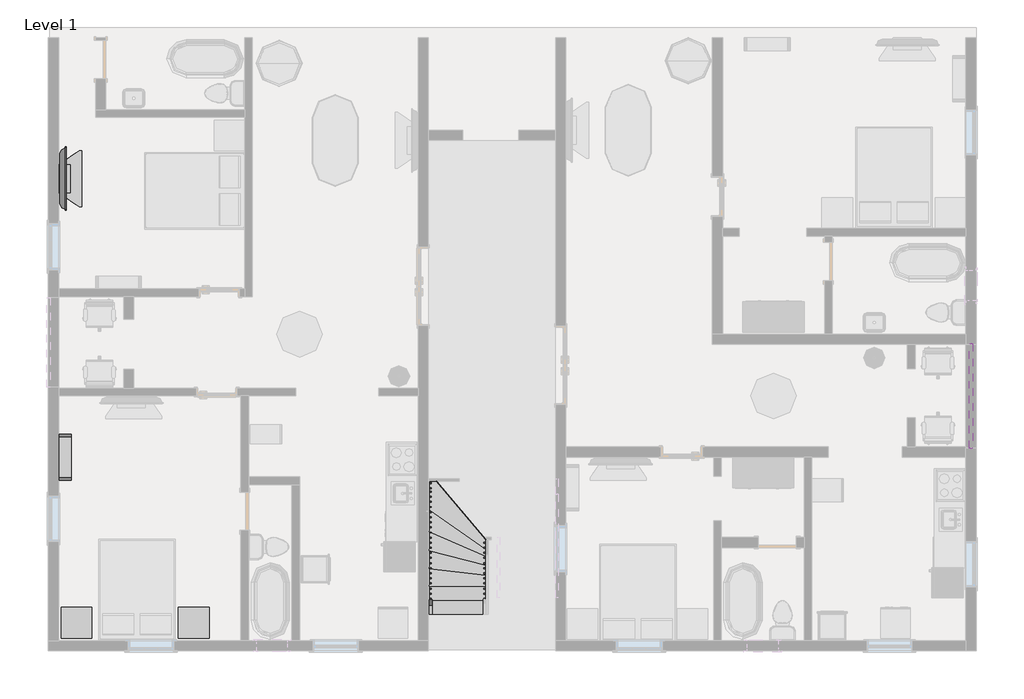
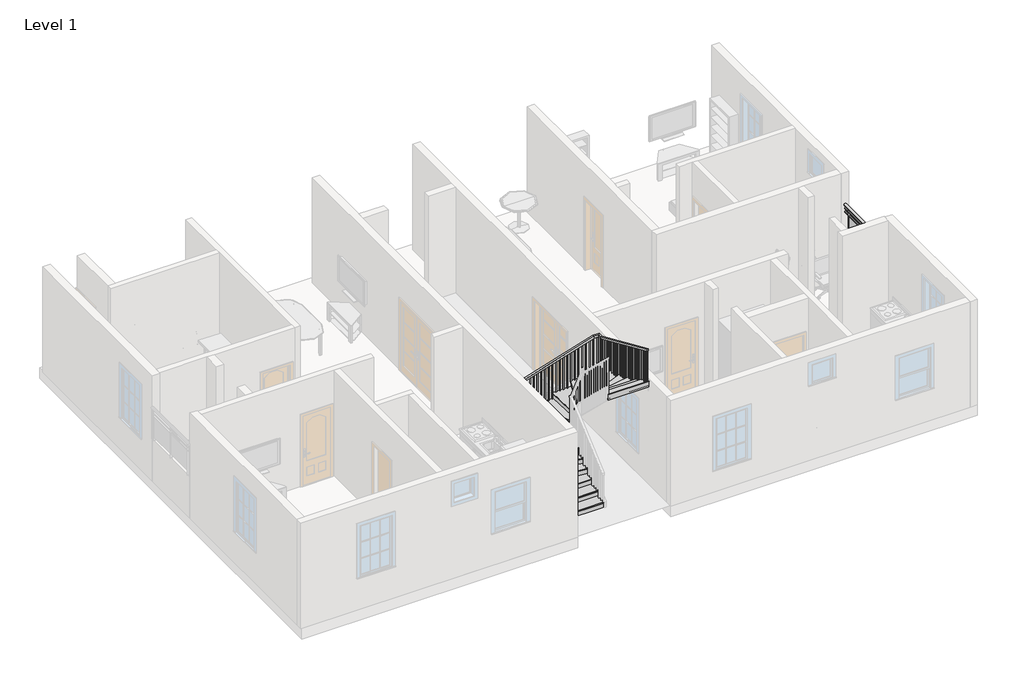
# One storey, part 3 of 4: 5 furniture elements, 2 railings, 1 stair flight.
"""IFC4 building model written with IfcOpenShell, lengths in millimetres."""

from ifc_helpers import new_model, si_unit, point, frame, origin, place, context, project, spatial, polyline, ellipse_curve, trimmed, outline, extrude, faceted_brep, transform, mapped, element, save
from ifc_brep_helpers import plane_surface, extruded_surface, advanced_brep
from components import furniture_417d203a, furniture_fdf74506, tv_stand_tv_stand_6ce107e5, furniture_5bc9ed15, stair_flight_2fadb1b5

model = new_model("IFC4")

# Units and contexts
model_context = context("Model", 3, world=origin())
ifc_project = project(units=[si_unit("LENGTHUNIT", "METRE", prefix="MILLI")], contexts=[model_context])

# Site, building, storey
site = spatial("IfcSite", under=ifc_project)
building = spatial("IfcBuilding", under=site)
storey = spatial("IfcBuildingStorey", under=building, Name="Level 1", Elevation=0.0)

# Furniture
placement = place(None, origin())
furniture_shape = furniture_417d203a(model_context)
element("IfcFurniture", 1, ObjectType="Shelving : 36\" x 10\" x 72\"", at=placement, inside=storey, context=model_context, shape_type="MappedRepresentation", body=[
    mapped(furniture_shape, transform((-16002.1808972, 4333.7923354, 0.0), x_axis=(0.0, -1.0000000000000004, 0.0), y_axis=(1.0000000000000004, 0.0, 0.0), z_axis=(0.0, 0.0, 1.0))),
])
furniture_2_shape = furniture_fdf74506(model_context)
element("IfcFurniture", 2, ObjectType="TV - Flat Screen : 50\"", at=placement, inside=storey, context=model_context, shape_type="MappedRepresentation", body=[
    mapped(furniture_2_shape, transform((-16350.6127714, 9887.6368496, 914.4), x_axis=(0.0, 0.9999999999999998, 0.0), y_axis=(-0.9999999999999998, 0.0, 0.0), z_axis=(0.0, 0.0, 1.0))),
])
tv_stand_tv_stand_shape = tv_stand_tv_stand_6ce107e5(model_context)
element("IfcFurniture", 3, ObjectType="TV Stand : TV Stand", at=placement, inside=storey, context=model_context, shape_type="MappedRepresentation", body=[
    mapped(tv_stand_tv_stand_shape, transform((-16433.9808972, 9758.5043334, 0.0), x_axis=(0.0, 1.0, 0.0), y_axis=(-1.0, 0.0, 0.0), z_axis=(0.0, 0.0, 1.0))),
])
furniture_3_shape = furniture_5bc9ed15(model_context)
element("IfcFurniture", 4, ObjectType="Table-Night Stand : 24\" x 24\" x 30\"", at=placement, inside=storey, context=model_context, shape_type="MappedRepresentation", body=[
    mapped(furniture_3_shape, transform((-14050.1145275, 726.9923354, 0.0), x_axis=(1.0, 0.0, 0.0), y_axis=(0.0, 1.0, 0.0), z_axis=(0.0, 0.0, 1.0))),
])
element("IfcFurniture", 5, ObjectType="Table-Night Stand : 24\" x 24\" x 30\"", at=placement, inside=storey, context=model_context, shape_type="MappedRepresentation", body=[
    mapped(furniture_3_shape, transform((-16386.9145275, 726.9923354, 0.0), x_axis=(1.0, 0.0, 0.0), y_axis=(0.0, 1.0, 0.0), z_axis=(0.0, 0.0, 1.0))),
])

# Railings
element("IfcRailing", 6, ObjectType="Glass Panel - Bottom Fill", at=placement, inside=storey, context=model_context, shape_type="SolidModel", body=[
    advanced_brep(
    [(1714.3191028, 4511.5923354, 2133.6), (1790.5191028, 4511.5923354, 2133.6), (1714.3191028, 6594.3923354, 2133.6), (1790.5191028, 6594.3923354, 2133.6)],
    [
        (0, 1, ellipse_curve(frame((1752.4191028, 4511.5923354, 2133.6), z_axis=(0.0, -1.0, 0.0), x_axis=(1.0, 0.0, 0.0)), 38.1, 28.575)),
        (1, 0, ellipse_curve(frame((1752.4191028, 4511.5923354, 2133.6), z_axis=(0.0, -1.0, 0.0), x_axis=(1.0, 0.0, 0.0)), 38.1, 28.575)),
        (2, 3, ellipse_curve(frame((1752.4191028, 6594.3923354, 2133.6), z_axis=(0.0, 1.0, 0.0), x_axis=(1.0, 0.0, 0.0)), 38.1, 28.575)),
        (3, 2, ellipse_curve(frame((1752.4191028, 6594.3923354, 2133.6), z_axis=(0.0, 1.0, 0.0), x_axis=(1.0, 0.0, 0.0)), 38.1, 28.575)),
        (0, 2),
        (3, 1),
    ],
    [
        plane_surface(frame((1752.4191028, 4511.5923354, 2133.6), z_axis=(0.0, -1.0, 0.0), x_axis=(0.0, 0.0, 1.0))),
        plane_surface(frame((1752.4191028, 6594.3923354, 2133.6), z_axis=(0.0, 1.0, 0.0), x_axis=(0.0, 0.0, 1.0))),
        extruded_surface(trimmed(ellipse_curve(frame((1752.4191028, 6594.3923354, 2133.6), z_axis=(0.0, -1.0, 0.0), x_axis=(1.0, 0.0, 0.0)), 38.1, 28.575), [point((1714.3191028, 6594.3923354, 2133.6))], [point((1790.5191028, 6594.3923354, 2133.6))], True, "CARTESIAN"), (0.0, -2082.8, 0.0), 2082.8),
        extruded_surface(trimmed(ellipse_curve(frame((1752.4191028, 6594.3923354, 2133.6), z_axis=(0.0, -1.0, 0.0), x_axis=(1.0, 0.0, 0.0)), 38.1, 28.575), [point((1790.5191028, 6594.3923354, 2133.6))], [point((1714.3191028, 6594.3923354, 2133.6))], True, "CARTESIAN"), (0.0, -2082.8, 0.0), 2082.8),
    ],
    [
        (0, [[1, 2]]),
        (1, [[3, 4]]),
        (2, [[-1, 5, -4, 6]]),
        (3, [[-2, -6, -3, -5]]),
    ],
),
    extrude(outline(polyline([(1765.1191028, 4511.5923354), (1739.7191028, 4511.5923354), (1739.7191028, 6594.3923354), (1765.1191028, 6594.3923354), (1765.1191028, 4511.5923354)])), frame((0.0, 0.0, 2019.3), z_axis=(0.0, 0.0, 1.0), x_axis=(1.0, 0.0, 0.0)), (0.0, 0.0, 1.0), 25.4),
    extrude(outline(polyline([(1765.1191028, 4511.5923354), (1739.7191028, 4511.5923354), (1739.7191028, 6594.3923354), (1765.1191028, 6594.3923354), (1765.1191028, 4511.5923354)])), frame((0.0, 0.0, 1917.7), z_axis=(0.0, 0.0, 1.0), x_axis=(1.0, 0.0, 0.0)), (0.0, 0.0, 1.0), 25.4),
    extrude(outline(polyline([(1777.8191028, 6359.4423354), (1727.0191028, 6359.4423354), (1727.0191028, 6372.1423354), (1777.8191028, 6372.1423354), (1777.8191028, 6359.4423354)])), frame((0.0, 0.0, 1219.2), z_axis=(0.0, 0.0, 1.0), x_axis=(1.0, 0.0, 0.0)), (0.0, 0.0, 1.0), 885.6788223),
    extrude(outline(polyline([(1745.8839458, 5552.9923354), (1745.8839458, 6365.7923354), (1752.2339458, 6365.7923354), (1752.2339458, 5552.9923354), (1745.8839458, 5552.9923354)])), frame((0.0, 0.0, 1320.8), z_axis=(0.0, 0.0, 1.0), x_axis=(1.0, 0.0, 0.0)), (0.0, 0.0, 1.0), 596.9),
    extrude(outline(polyline([(1777.8191028, 5546.6423354), (1727.0191028, 5546.6423354), (1727.0191028, 5559.3423354), (1777.8191028, 5559.3423354), (1777.8191028, 5546.6423354)])), frame((0.0, 0.0, 1219.2), z_axis=(0.0, 0.0, 1.0), x_axis=(1.0, 0.0, 0.0)), (0.0, 0.0, 1.0), 885.6788223),
    extrude(outline(polyline([(1745.8839458, 4740.1923354), (1745.8839458, 5552.9923354), (1752.2339458, 5552.9923354), (1752.2339458, 4740.1923354), (1745.8839458, 4740.1923354)])), frame((0.0, 0.0, 1320.8), z_axis=(0.0, 0.0, 1.0), x_axis=(1.0, 0.0, 0.0)), (0.0, 0.0, 1.0), 596.9),
    extrude(outline(polyline([(1777.8191028, 4733.8423354), (1727.0191028, 4733.8423354), (1727.0191028, 4746.5423354), (1777.8191028, 4746.5423354), (1777.8191028, 4733.8423354)])), frame((0.0, 0.0, 1219.2), z_axis=(0.0, 0.0, 1.0), x_axis=(1.0, 0.0, 0.0)), (0.0, 0.0, 1.0), 885.6788223),
    extrude(outline(polyline([(1761.9441028, 6581.6923354), (1742.8941028, 6581.6923354), (1742.8941028, 6600.7423354), (1761.9441028, 6600.7423354), (1761.9441028, 6581.6923354)])), frame((0.0, 0.0, 1219.2), z_axis=(0.0, 0.0, 1.0), x_axis=(1.0, 0.0, 0.0)), (0.0, 0.0, 1.0), 885.6788223),
    extrude(outline(polyline([(1761.9441028, 4505.2423354), (1742.8941028, 4505.2423354), (1742.8941028, 4524.2923354), (1761.9441028, 4524.2923354), (1761.9441028, 4505.2423354)])), frame((0.0, 0.0, 1219.2), z_axis=(0.0, 0.0, 1.0), x_axis=(1.0, 0.0, 0.0)), (0.0, 0.0, 1.0), 885.6788223),
])
element("IfcRailing", 7, ObjectType="Handrail - Rectangular", at=placement, inside=storey, context=model_context, shape_type="SolidModel", body=[
    faceted_brep([(-9042.5808972, 1205.8606436, 1121.9367255), (-9042.5808972, 1205.8606436, 1065.8201346), (-8991.7808972, 1205.8606436, 1065.8201346), (-8991.7808972, 1205.8606436, 1121.9367255), (-9042.5808972, 3713.0769303, 2298.6408203), (-9042.5808972, 3724.4050489, 2247.8408203), (-8991.7808972, 3724.4050489, 2247.8408203), (-8991.7808972, 3713.0769303, 2298.6408203), (-9042.5808972, 3851.1923354, 2298.6408203), (-9042.5808972, 3851.1923354, 2247.8408203), (-8991.7808972, 3800.3923354, 2247.8408203), (-8991.7808972, 3800.3923354, 2298.6408203), (-8844.6177246, 3851.1923354, 2298.6408203), (-8837.0060044, 3851.1923354, 2247.8408203), (-8837.0060044, 3800.3923354, 2247.8408203), (-8844.6177246, 3800.3923354, 2298.6408203), (-6708.6398439, 3851.1923354, 2953.4388666), (-6701.0281237, 3851.1923354, 2902.6388666), (-6701.0281237, 3800.3923354, 2902.6388666), (-6708.6398439, 3800.3923354, 2953.4388666), (-6527.9808972, 3851.1923354, 2953.4388666), (-6527.9808972, 3851.1923354, 2902.6388666), (-6578.7808972, 3800.3923354, 2902.6388666), (-6578.7808972, 3800.3923354, 2953.4388666), (-6527.9808972, 3717.5997251, 2953.4388666), (-6527.9808972, 3706.9197367, 2902.6388666), (-6578.7808972, 3706.9197367, 2902.6388666), (-6578.7808972, 3717.5997251, 2953.4388666), (-6527.9808972, 1529.5899254, 3915.9791695), (-6578.7808972, 1529.5899254, 3915.9791695), (-6578.7808972, 1529.5899254, 3860.4808728), (-6527.9808972, 1529.5899254, 3860.4808728)], [[[0, 1, 2, 3]], [[1, 0, 4, 5]], [[2, 1, 5, 6]], [[3, 2, 6, 7]], [[0, 3, 7, 4]], [[5, 4, 8, 9]], [[6, 5, 9, 10]], [[7, 6, 10, 11]], [[4, 7, 11, 8]], [[9, 8, 12, 13]], [[10, 9, 13, 14]], [[11, 10, 14, 15]], [[8, 11, 15, 12]], [[13, 12, 16, 17]], [[14, 13, 17, 18]], [[15, 14, 18, 19]], [[12, 15, 19, 16]], [[17, 16, 20, 21]], [[18, 17, 21, 22]], [[19, 18, 22, 23]], [[16, 19, 23, 20]], [[21, 20, 24, 25]], [[22, 21, 25, 26]], [[23, 22, 26, 27]], [[20, 23, 27, 24]], [[28, 29, 30, 31]], [[25, 24, 28, 31]], [[26, 25, 31, 30]], [[27, 26, 30, 29]], [[24, 27, 29, 28]]]),
    extrude(outline(polyline([(1593.5247251, 3832.3549378), (1593.5247251, 2878.6666667), (1574.4747251, 2878.6666667), (1574.4747251, 3840.7353357), (1593.5247251, 3832.3549378)])), frame((-6562.9058972, 0.0, 0.0), z_axis=(1.0, 0.0, 0.0), x_axis=(0.0, 1.0, 0.0)), (0.0, 0.0, 1.0), 19.05),
    extrude(outline(polyline([(1695.1247251, 3787.6594822), (1695.1247251, 2878.6666667), (1676.0747251, 2878.6666667), (1676.0747251, 3796.0398801), (1695.1247251, 3787.6594822)])), frame((-6562.9058972, 0.0, 0.0), z_axis=(1.0, 0.0, 0.0), x_axis=(0.0, 1.0, 0.0)), (0.0, 0.0, 1.0), 19.05),
    extrude(outline(polyline([(1796.7247251, 3742.9640266), (1796.7247251, 2878.6666667), (1777.6747251, 2878.6666667), (1777.6747251, 3751.3444246), (1796.7247251, 3742.9640266)])), frame((-6562.9058972, 0.0, 0.0), z_axis=(1.0, 0.0, 0.0), x_axis=(0.0, 1.0, 0.0)), (0.0, 0.0, 1.0), 19.05),
    extrude(outline(polyline([(1898.3247251, 3698.2685711), (1898.3247251, 2709.3333333), (1879.2747251, 2709.3333333), (1879.2747251, 3706.648969), (1898.3247251, 3698.2685711)])), frame((-6562.9058972, 0.0, 0.0), z_axis=(1.0, 0.0, 0.0), x_axis=(0.0, 1.0, 0.0)), (0.0, 0.0, 1.0), 19.05),
    extrude(outline(polyline([(1999.9247251, 3653.5731155), (1999.9247251, 2709.3333333), (1980.8747251, 2709.3333333), (1980.8747251, 3661.9535134), (1999.9247251, 3653.5731155)])), frame((-6562.9058972, 0.0, 0.0), z_axis=(1.0, 0.0, 0.0), x_axis=(0.0, 1.0, 0.0)), (0.0, 0.0, 1.0), 19.05),
    extrude(outline(polyline([(2101.5247251, 3608.8776599), (2101.5247251, 2540.0), (2082.4747251, 2540.0), (2082.4747251, 3617.2580579), (2101.5247251, 3608.8776599)])), frame((-6562.9058972, 0.0, 0.0), z_axis=(1.0, 0.0, 0.0), x_axis=(0.0, 1.0, 0.0)), (0.0, 0.0, 1.0), 19.05),
    extrude(outline(polyline([(2203.1247251, 3564.1822044), (2203.1247251, 2540.0), (2184.0747251, 2540.0), (2184.0747251, 3572.5626023), (2203.1247251, 3564.1822044)])), frame((-6562.9058972, 0.0, 0.0), z_axis=(1.0, 0.0, 0.0), x_axis=(0.0, 1.0, 0.0)), (0.0, 0.0, 1.0), 19.05),
    extrude(outline(polyline([(2304.7247251, 3519.4867488), (2304.7247251, 2540.0), (2285.6747251, 2540.0), (2285.6747251, 3527.8671467), (2304.7247251, 3519.4867488)])), frame((-6562.9058972, 0.0, 0.0), z_axis=(1.0, 0.0, 0.0), x_axis=(0.0, 1.0, 0.0)), (0.0, 0.0, 1.0), 19.05),
    extrude(outline(polyline([(2406.3247251, 3474.7912933), (2406.3247251, 2540.0), (2387.2747251, 2540.0), (2387.2747251, 3483.1716912), (2406.3247251, 3474.7912933)])), frame((-6562.9058972, 0.0, 0.0), z_axis=(1.0, 0.0, 0.0), x_axis=(0.0, 1.0, 0.0)), (0.0, 0.0, 1.0), 19.05),
    extrude(outline(polyline([(2507.9247251, 3430.0958377), (2507.9247251, 2370.6666667), (2488.8747251, 2370.6666667), (2488.8747251, 3438.4762356), (2507.9247251, 3430.0958377)])), frame((-6562.9058972, 0.0, 0.0), z_axis=(1.0, 0.0, 0.0), x_axis=(0.0, 1.0, 0.0)), (0.0, 0.0, 1.0), 19.05),
    extrude(outline(polyline([(2609.5247251, 3385.4003821), (2609.5247251, 2370.6666667), (2590.4747251, 2370.6666667), (2590.4747251, 3393.78078), (2609.5247251, 3385.4003821)])), frame((-6562.9058972, 0.0, 0.0), z_axis=(1.0, 0.0, 0.0), x_axis=(0.0, 1.0, 0.0)), (0.0, 0.0, 1.0), 19.05),
    extrude(outline(polyline([(2711.1247251, 3340.7049266), (2711.1247251, 2370.6666667), (2692.0747251, 2370.6666667), (2692.0747251, 3349.0853245), (2711.1247251, 3340.7049266)])), frame((-6562.9058972, 0.0, 0.0), z_axis=(1.0, 0.0, 0.0), x_axis=(0.0, 1.0, 0.0)), (0.0, 0.0, 1.0), 19.05),
    extrude(outline(polyline([(2812.7247251, 3296.009471), (2812.7247251, 2370.6666667), (2793.6747251, 2370.6666667), (2793.6747251, 3304.3898689), (2812.7247251, 3296.009471)])), frame((-6562.9058972, 0.0, 0.0), z_axis=(1.0, 0.0, 0.0), x_axis=(0.0, 1.0, 0.0)), (0.0, 0.0, 1.0), 19.05),
    extrude(outline(polyline([(2914.3247251, 3251.3140154), (2914.3247251, 2201.3333333), (2895.2747251, 2201.3333333), (2895.2747251, 3259.6944134), (2914.3247251, 3251.3140154)])), frame((-6562.9058972, 0.0, 0.0), z_axis=(1.0, 0.0, 0.0), x_axis=(0.0, 1.0, 0.0)), (0.0, 0.0, 1.0), 19.05),
    extrude(outline(polyline([(3015.9247251, 3206.6185599), (3015.9247251, 2201.3333333), (2996.8747251, 2201.3333333), (2996.8747251, 3214.9989578), (3015.9247251, 3206.6185599)])), frame((-6562.9058972, 0.0, 0.0), z_axis=(1.0, 0.0, 0.0), x_axis=(0.0, 1.0, 0.0)), (0.0, 0.0, 1.0), 19.05),
    extrude(outline(polyline([(3117.5247251, 3161.9231043), (3117.5247251, 2201.3333333), (3098.4747251, 2201.3333333), (3098.4747251, 3170.3035022), (3117.5247251, 3161.9231043)])), frame((-6562.9058972, 0.0, 0.0), z_axis=(1.0, 0.0, 0.0), x_axis=(0.0, 1.0, 0.0)), (0.0, 0.0, 1.0), 19.05),
    extrude(outline(polyline([(3219.1247251, 3117.2276487), (3219.1247251, 2201.3333333), (3200.0747251, 2201.3333333), (3200.0747251, 3125.6080467), (3219.1247251, 3117.2276487)])), frame((-6562.9058972, 0.0, 0.0), z_axis=(1.0, 0.0, 0.0), x_axis=(0.0, 1.0, 0.0)), (0.0, 0.0, 1.0), 19.05),
    extrude(outline(polyline([(3320.7247251, 3072.5321932), (3320.7247251, 2201.3333333), (3301.6747251, 2201.3333333), (3301.6747251, 3080.9125911), (3320.7247251, 3072.5321932)])), frame((-6562.9058972, 0.0, 0.0), z_axis=(1.0, 0.0, 0.0), x_axis=(0.0, 1.0, 0.0)), (0.0, 0.0, 1.0), 19.05),
    extrude(outline(polyline([(3422.3247251, 3027.8367376), (3422.3247251, 2032.0), (3403.2747251, 2032.0), (3403.2747251, 3036.2171355), (3422.3247251, 3027.8367376)])), frame((-6562.9058972, 0.0, 0.0), z_axis=(1.0, 0.0, 0.0), x_axis=(0.0, 1.0, 0.0)), (0.0, 0.0, 1.0), 19.05),
    extrude(outline(polyline([(3523.9247251, 2983.1412821), (3523.9247251, 2032.0), (3504.8747251, 2032.0), (3504.8747251, 2991.52168), (3523.9247251, 2983.1412821)])), frame((-6562.9058972, 0.0, 0.0), z_axis=(1.0, 0.0, 0.0), x_axis=(0.0, 1.0, 0.0)), (0.0, 0.0, 1.0), 19.05),
    extrude(outline(polyline([(3625.5247251, 2938.4458265), (3625.5247251, 2032.0), (3606.4747251, 2032.0), (3606.4747251, 2946.8262244), (3625.5247251, 2938.4458265)])), frame((-6562.9058972, 0.0, 0.0), z_axis=(1.0, 0.0, 0.0), x_axis=(0.0, 1.0, 0.0)), (0.0, 0.0, 1.0), 19.05),
    extrude(outline(polyline([(-6543.8558972, 3733.7173354), (-6543.8558972, 3714.6673354), (-6562.9058972, 3714.6673354), (-6562.9058972, 3733.7173354), (-6543.8558972, 3733.7173354)])), frame((0.0, 0.0, 2032.0), z_axis=(0.0, 0.0, 1.0), x_axis=(1.0, 0.0, 0.0)), (0.0, 0.0, 1.0), 870.6388666),
    extrude(outline(polyline([(-6616.5648439, 3835.3173354), (-6597.5148439, 3835.3173354), (-6597.5148439, 3816.2673354), (-6616.5648439, 3816.2673354), (-6616.5648439, 3835.3173354)])), frame((0.0, 0.0, 2032.0), z_axis=(0.0, 0.0, 1.0), x_axis=(1.0, 0.0, 0.0)), (0.0, 0.0, 1.0), 870.6388666),
    extrude(outline(polyline([(2896.6565375, -6720.5427246), (2032.0, -6720.5427246), (2032.0, -6701.4927246), (2902.4964401, -6701.4927246), (2896.6565375, -6720.5427246)])), frame((0.0, 3816.2673354, 0.0), z_axis=(0.0, 1.0, 0.0), x_axis=(0.0, 0.0, 1.0)), (0.0, 0.0, 1.0), 19.05),
    extrude(outline(polyline([(2865.5103903, -6822.1427246), (1862.6666667, -6822.1427246), (1862.6666667, -6803.0927246), (2871.3502929, -6803.0927246), (2865.5103903, -6822.1427246)])), frame((0.0, 3816.2673354, 0.0), z_axis=(0.0, 1.0, 0.0), x_axis=(0.0, 0.0, 1.0)), (0.0, 0.0, 1.0), 19.05),
    extrude(outline(polyline([(2834.3642431, -6923.7427246), (1862.6666667, -6923.7427246), (1862.6666667, -6904.6927246), (2840.2041457, -6904.6927246), (2834.3642431, -6923.7427246)])), frame((0.0, 3816.2673354, 0.0), z_axis=(0.0, 1.0, 0.0), x_axis=(0.0, 0.0, 1.0)), (0.0, 0.0, 1.0), 19.05),
    extrude(outline(polyline([(2803.2180959, -7025.3427246), (1862.6666667, -7025.3427246), (1862.6666667, -7006.2927246), (2809.0579985, -7006.2927246), (2803.2180959, -7025.3427246)])), frame((0.0, 3816.2673354, 0.0), z_axis=(0.0, 1.0, 0.0), x_axis=(0.0, 0.0, 1.0)), (0.0, 0.0, 1.0), 19.05),
    extrude(outline(polyline([(2772.0719487, -7126.9427246), (1862.6666667, -7126.9427246), (1862.6666667, -7107.8927246), (2777.9118513, -7107.8927246), (2772.0719487, -7126.9427246)])), frame((0.0, 3816.2673354, 0.0), z_axis=(0.0, 1.0, 0.0), x_axis=(0.0, 0.0, 1.0)), (0.0, 0.0, 1.0), 19.05),
    extrude(outline(polyline([(2740.9258015, -7228.5427246), (1862.6666667, -7228.5427246), (1862.6666667, -7209.4927246), (2746.7657041, -7209.4927246), (2740.9258015, -7228.5427246)])), frame((0.0, 3816.2673354, 0.0), z_axis=(0.0, 1.0, 0.0), x_axis=(0.0, 0.0, 1.0)), (0.0, 0.0, 1.0), 19.05),
    extrude(outline(polyline([(2709.7796543, -7330.1427246), (1862.6666667, -7330.1427246), (1862.6666667, -7311.0927246), (2715.6195569, -7311.0927246), (2709.7796543, -7330.1427246)])), frame((0.0, 3816.2673354, 0.0), z_axis=(0.0, 1.0, 0.0), x_axis=(0.0, 0.0, 1.0)), (0.0, 0.0, 1.0), 19.05),
    extrude(outline(polyline([(2678.6335071, -7431.7427246), (1693.3333333, -7431.7427246), (1693.3333333, -7412.6927246), (2684.4734097, -7412.6927246), (2678.6335071, -7431.7427246)])), frame((0.0, 3816.2673354, 0.0), z_axis=(0.0, 1.0, 0.0), x_axis=(0.0, 0.0, 1.0)), (0.0, 0.0, 1.0), 19.05),
    extrude(outline(polyline([(2647.4873599, -7533.3427246), (1693.3333333, -7533.3427246), (1693.3333333, -7514.2927246), (2653.3272625, -7514.2927246), (2647.4873599, -7533.3427246)])), frame((0.0, 3816.2673354, 0.0), z_axis=(0.0, 1.0, 0.0), x_axis=(0.0, 0.0, 1.0)), (0.0, 0.0, 1.0), 19.05),
    extrude(outline(polyline([(2616.3412127, -7634.9427246), (1693.3333333, -7634.9427246), (1693.3333333, -7615.8927246), (2622.1811153, -7615.8927246), (2616.3412127, -7634.9427246)])), frame((0.0, 3816.2673354, 0.0), z_axis=(0.0, 1.0, 0.0), x_axis=(0.0, 0.0, 1.0)), (0.0, 0.0, 1.0), 19.05),
    extrude(outline(polyline([(2585.1950655, -7736.5427246), (1693.3333333, -7736.5427246), (1693.3333333, -7717.4927246), (2591.0349681, -7717.4927246), (2585.1950655, -7736.5427246)])), frame((0.0, 3816.2673354, 0.0), z_axis=(0.0, 1.0, 0.0), x_axis=(0.0, 0.0, 1.0)), (0.0, 0.0, 1.0), 19.05),
    extrude(outline(polyline([(2554.0489183, -7838.1427246), (1524.0, -7838.1427246), (1524.0, -7819.0927246), (2559.8888209, -7819.0927246), (2554.0489183, -7838.1427246)])), frame((0.0, 3816.2673354, 0.0), z_axis=(0.0, 1.0, 0.0), x_axis=(0.0, 0.0, 1.0)), (0.0, 0.0, 1.0), 19.05),
    extrude(outline(polyline([(2522.902771, -7939.7427246), (1524.0, -7939.7427246), (1524.0, -7920.6927246), (2528.7426736, -7920.6927246), (2522.902771, -7939.7427246)])), frame((0.0, 3816.2673354, 0.0), z_axis=(0.0, 1.0, 0.0), x_axis=(0.0, 0.0, 1.0)), (0.0, 0.0, 1.0), 19.05),
    extrude(outline(polyline([(2491.7566238, -8041.3427246), (1524.0, -8041.3427246), (1524.0, -8022.2927246), (2497.5965264, -8022.2927246), (2491.7566238, -8041.3427246)])), frame((0.0, 3816.2673354, 0.0), z_axis=(0.0, 1.0, 0.0), x_axis=(0.0, 0.0, 1.0)), (0.0, 0.0, 1.0), 19.05),
    extrude(outline(polyline([(2460.6104766, -8142.9427246), (1524.0, -8142.9427246), (1524.0, -8123.8927246), (2466.4503792, -8123.8927246), (2460.6104766, -8142.9427246)])), frame((0.0, 3816.2673354, 0.0), z_axis=(0.0, 1.0, 0.0), x_axis=(0.0, 0.0, 1.0)), (0.0, 0.0, 1.0), 19.05),
    extrude(outline(polyline([(2429.4643294, -8244.5427246), (1524.0, -8244.5427246), (1524.0, -8225.4927246), (2435.304232, -8225.4927246), (2429.4643294, -8244.5427246)])), frame((0.0, 3816.2673354, 0.0), z_axis=(0.0, 1.0, 0.0), x_axis=(0.0, 0.0, 1.0)), (0.0, 0.0, 1.0), 19.05),
    extrude(outline(polyline([(2398.3181822, -8346.1427246), (1354.6666667, -8346.1427246), (1354.6666667, -8327.0927246), (2404.1580848, -8327.0927246), (2398.3181822, -8346.1427246)])), frame((0.0, 3816.2673354, 0.0), z_axis=(0.0, 1.0, 0.0), x_axis=(0.0, 0.0, 1.0)), (0.0, 0.0, 1.0), 19.05),
    extrude(outline(polyline([(2367.172035, -8447.7427246), (1354.6666667, -8447.7427246), (1354.6666667, -8428.6927246), (2373.0119376, -8428.6927246), (2367.172035, -8447.7427246)])), frame((0.0, 3816.2673354, 0.0), z_axis=(0.0, 1.0, 0.0), x_axis=(0.0, 0.0, 1.0)), (0.0, 0.0, 1.0), 19.05),
    extrude(outline(polyline([(2336.0258878, -8549.3427246), (1354.6666667, -8549.3427246), (1354.6666667, -8530.2927246), (2341.8657904, -8530.2927246), (2336.0258878, -8549.3427246)])), frame((0.0, 3816.2673354, 0.0), z_axis=(0.0, 1.0, 0.0), x_axis=(0.0, 0.0, 1.0)), (0.0, 0.0, 1.0), 19.05),
    extrude(outline(polyline([(2304.8797406, -8650.9427246), (1354.6666667, -8650.9427246), (1354.6666667, -8631.8927246), (2310.7196432, -8631.8927246), (2304.8797406, -8650.9427246)])), frame((0.0, 3816.2673354, 0.0), z_axis=(0.0, 1.0, 0.0), x_axis=(0.0, 0.0, 1.0)), (0.0, 0.0, 1.0), 19.05),
    extrude(outline(polyline([(2273.7335934, -8752.5427246), (1354.6666667, -8752.5427246), (1354.6666667, -8733.4927246), (2279.573496, -8733.4927246), (2273.7335934, -8752.5427246)])), frame((0.0, 3816.2673354, 0.0), z_axis=(0.0, 1.0, 0.0), x_axis=(0.0, 0.0, 1.0)), (0.0, 0.0, 1.0), 19.05),
    extrude(outline(polyline([(-8925.1058972, 3835.3173354), (-8906.0558972, 3835.3173354), (-8906.0558972, 3816.2673354), (-8925.1058972, 3816.2673354), (-8925.1058972, 3835.3173354)])), frame((0.0, 0.0, 1354.6666667), z_axis=(0.0, 0.0, 1.0), x_axis=(1.0, 0.0, 0.0)), (0.0, 0.0, 1.0), 893.1741537),
    extrude(outline(polyline([(-9026.7058972, 3805.1519303), (-9026.7058972, 3824.2019303), (-9007.6558972, 3824.2019303), (-9007.6558972, 3805.1519303), (-9026.7058972, 3805.1519303)])), frame((0.0, 0.0, 1185.3333333), z_axis=(0.0, 0.0, 1.0), x_axis=(1.0, 0.0, 0.0)), (0.0, 0.0, 1.0), 1062.507487),
    extrude(outline(polyline([(3653.7856436, 2214.6972324), (3653.7856436, 1185.3333333), (3634.7356436, 1185.3333333), (3634.7356436, 2205.7565546), (3653.7856436, 2214.6972324)])), frame((-9026.7058972, 0.0, 0.0), z_axis=(1.0, 0.0, 0.0), x_axis=(0.0, 1.0, 0.0)), (0.0, 0.0, 1.0), 19.05),
    extrude(outline(polyline([(3552.1856436, 2167.0136174), (3552.1856436, 1185.3333333), (3533.1356436, 1185.3333333), (3533.1356436, 2158.0729396), (3552.1856436, 2167.0136174)])), frame((-9026.7058972, 0.0, 0.0), z_axis=(1.0, 0.0, 0.0), x_axis=(0.0, 1.0, 0.0)), (0.0, 0.0, 1.0), 19.05),
    extrude(outline(polyline([(3450.5856436, 2119.3300025), (3450.5856436, 1185.3333333), (3431.5356436, 1185.3333333), (3431.5356436, 2110.3893247), (3450.5856436, 2119.3300025)])), frame((-9026.7058972, 0.0, 0.0), z_axis=(1.0, 0.0, 0.0), x_axis=(0.0, 1.0, 0.0)), (0.0, 0.0, 1.0), 19.05),
    extrude(outline(polyline([(3348.9856436, 2071.6463875), (3348.9856436, 1185.3333333), (3329.9356436, 1185.3333333), (3329.9356436, 2062.7057097), (3348.9856436, 2071.6463875)])), frame((-9026.7058972, 0.0, 0.0), z_axis=(1.0, 0.0, 0.0), x_axis=(0.0, 1.0, 0.0)), (0.0, 0.0, 1.0), 19.05),
    extrude(outline(polyline([(3247.3856436, 2023.9627726), (3247.3856436, 1016.0), (3228.3356436, 1016.0), (3228.3356436, 2015.0220948), (3247.3856436, 2023.9627726)])), frame((-9026.7058972, 0.0, 0.0), z_axis=(1.0, 0.0, 0.0), x_axis=(0.0, 1.0, 0.0)), (0.0, 0.0, 1.0), 19.05),
    extrude(outline(polyline([(3145.7856436, 1976.2791576), (3145.7856436, 1016.0), (3126.7356436, 1016.0), (3126.7356436, 1967.3384798), (3145.7856436, 1976.2791576)])), frame((-9026.7058972, 0.0, 0.0), z_axis=(1.0, 0.0, 0.0), x_axis=(0.0, 1.0, 0.0)), (0.0, 0.0, 1.0), 19.05),
    extrude(outline(polyline([(3044.1856436, 1928.5955427), (3044.1856436, 1016.0), (3025.1356436, 1016.0), (3025.1356436, 1919.6548649), (3044.1856436, 1928.5955427)])), frame((-9026.7058972, 0.0, 0.0), z_axis=(1.0, 0.0, 0.0), x_axis=(0.0, 1.0, 0.0)), (0.0, 0.0, 1.0), 19.05),
    extrude(outline(polyline([(2942.5856436, 1880.9119277), (2942.5856436, 1016.0), (2923.5356436, 1016.0), (2923.5356436, 1871.9712499), (2942.5856436, 1880.9119277)])), frame((-9026.7058972, 0.0, 0.0), z_axis=(1.0, 0.0, 0.0), x_axis=(0.0, 1.0, 0.0)), (0.0, 0.0, 1.0), 19.05),
    extrude(outline(polyline([(2840.9856436, 1833.2283128), (2840.9856436, 846.6666667), (2821.9356436, 846.6666667), (2821.9356436, 1824.2876349), (2840.9856436, 1833.2283128)])), frame((-9026.7058972, 0.0, 0.0), z_axis=(1.0, 0.0, 0.0), x_axis=(0.0, 1.0, 0.0)), (0.0, 0.0, 1.0), 19.05),
    extrude(outline(polyline([(2739.3856436, 1785.5446978), (2739.3856436, 846.6666667), (2720.3356436, 846.6666667), (2720.3356436, 1776.60402), (2739.3856436, 1785.5446978)])), frame((-9026.7058972, 0.0, 0.0), z_axis=(1.0, 0.0, 0.0), x_axis=(0.0, 1.0, 0.0)), (0.0, 0.0, 1.0), 19.05),
    extrude(outline(polyline([(2637.7856436, 1737.8610828), (2637.7856436, 846.6666667), (2618.7356436, 846.6666667), (2618.7356436, 1728.920405), (2637.7856436, 1737.8610828)])), frame((-9026.7058972, 0.0, 0.0), z_axis=(1.0, 0.0, 0.0), x_axis=(0.0, 1.0, 0.0)), (0.0, 0.0, 1.0), 19.05),
    extrude(outline(polyline([(2536.1856436, 1690.1774679), (2536.1856436, 846.6666667), (2517.1356436, 846.6666667), (2517.1356436, 1681.2367901), (2536.1856436, 1690.1774679)])), frame((-9026.7058972, 0.0, 0.0), z_axis=(1.0, 0.0, 0.0), x_axis=(0.0, 1.0, 0.0)), (0.0, 0.0, 1.0), 19.05),
    extrude(outline(polyline([(2434.5856436, 1642.4938529), (2434.5856436, 677.3333333), (2415.5356436, 677.3333333), (2415.5356436, 1633.5531751), (2434.5856436, 1642.4938529)])), frame((-9026.7058972, 0.0, 0.0), z_axis=(1.0, 0.0, 0.0), x_axis=(0.0, 1.0, 0.0)), (0.0, 0.0, 1.0), 19.05),
    extrude(outline(polyline([(2332.9856436, 1594.810238), (2332.9856436, 677.3333333), (2313.9356436, 677.3333333), (2313.9356436, 1585.8695602), (2332.9856436, 1594.810238)])), frame((-9026.7058972, 0.0, 0.0), z_axis=(1.0, 0.0, 0.0), x_axis=(0.0, 1.0, 0.0)), (0.0, 0.0, 1.0), 19.05),
    extrude(outline(polyline([(2231.3856436, 1547.126623), (2231.3856436, 677.3333333), (2212.3356436, 677.3333333), (2212.3356436, 1538.1859452), (2231.3856436, 1547.126623)])), frame((-9026.7058972, 0.0, 0.0), z_axis=(1.0, 0.0, 0.0), x_axis=(0.0, 1.0, 0.0)), (0.0, 0.0, 1.0), 19.05),
    extrude(outline(polyline([(2129.7856436, 1499.4430081), (2129.7856436, 677.3333333), (2110.7356436, 677.3333333), (2110.7356436, 1490.5023303), (2129.7856436, 1499.4430081)])), frame((-9026.7058972, 0.0, 0.0), z_axis=(1.0, 0.0, 0.0), x_axis=(0.0, 1.0, 0.0)), (0.0, 0.0, 1.0), 19.05),
    extrude(outline(polyline([(2028.1856436, 1451.7593931), (2028.1856436, 508.0), (2009.1356436, 508.0), (2009.1356436, 1442.8187153), (2028.1856436, 1451.7593931)])), frame((-9026.7058972, 0.0, 0.0), z_axis=(1.0, 0.0, 0.0), x_axis=(0.0, 1.0, 0.0)), (0.0, 0.0, 1.0), 19.05),
    extrude(outline(polyline([(1926.5856436, 1404.0757781), (1926.5856436, 508.0), (1907.5356436, 508.0), (1907.5356436, 1395.1351003), (1926.5856436, 1404.0757781)])), frame((-9026.7058972, 0.0, 0.0), z_axis=(1.0, 0.0, 0.0), x_axis=(0.0, 1.0, 0.0)), (0.0, 0.0, 1.0), 19.05),
    extrude(outline(polyline([(1824.9856436, 1356.3921632), (1824.9856436, 508.0), (1805.9356436, 508.0), (1805.9356436, 1347.4514854), (1824.9856436, 1356.3921632)])), frame((-9026.7058972, 0.0, 0.0), z_axis=(1.0, 0.0, 0.0), x_axis=(0.0, 1.0, 0.0)), (0.0, 0.0, 1.0), 19.05),
    extrude(outline(polyline([(1723.3856436, 1308.7085482), (1723.3856436, 338.6666667), (1704.3356436, 338.6666667), (1704.3356436, 1299.7678704), (1723.3856436, 1308.7085482)])), frame((-9026.7058972, 0.0, 0.0), z_axis=(1.0, 0.0, 0.0), x_axis=(0.0, 1.0, 0.0)), (0.0, 0.0, 1.0), 19.05),
    extrude(outline(polyline([(1621.7856436, 1261.0249333), (1621.7856436, 338.6666667), (1602.7356436, 338.6666667), (1602.7356436, 1252.0842555), (1621.7856436, 1261.0249333)])), frame((-9026.7058972, 0.0, 0.0), z_axis=(1.0, 0.0, 0.0), x_axis=(0.0, 1.0, 0.0)), (0.0, 0.0, 1.0), 19.05),
    extrude(outline(polyline([(1520.1856436, 1213.3413183), (1520.1856436, 338.6666667), (1501.1356436, 338.6666667), (1501.1356436, 1204.4006405), (1520.1856436, 1213.3413183)])), frame((-9026.7058972, 0.0, 0.0), z_axis=(1.0, 0.0, 0.0), x_axis=(0.0, 1.0, 0.0)), (0.0, 0.0, 1.0), 19.05),
    extrude(outline(polyline([(1418.5856436, 1165.6577034), (1418.5856436, 169.3333333), (1399.5356436, 169.3333333), (1399.5356436, 1156.7170256), (1418.5856436, 1165.6577034)])), frame((-9026.7058972, 0.0, 0.0), z_axis=(1.0, 0.0, 0.0), x_axis=(0.0, 1.0, 0.0)), (0.0, 0.0, 1.0), 19.05),
    extrude(outline(polyline([(1316.9856436, 1117.9740884), (1316.9856436, 169.3333333), (1297.9356436, 169.3333333), (1297.9356436, 1109.0334106), (1316.9856436, 1117.9740884)])), frame((-9026.7058972, 0.0, 0.0), z_axis=(1.0, 0.0, 0.0), x_axis=(0.0, 1.0, 0.0)), (0.0, 0.0, 1.0), 19.05),
    extrude(outline(polyline([(-6543.8558972, 3727.1247251), (-6543.8558972, 3708.0747251), (-6562.9058972, 3708.0747251), (-6562.9058972, 3727.1247251), (-6543.8558972, 3727.1247251)])), frame((0.0, 0.0, 2032.0), z_axis=(0.0, 0.0, 1.0), x_axis=(1.0, 0.0, 0.0)), (0.0, 0.0, 1.0), 870.6388666),
    extrude(outline(polyline([(-6562.9058972, 3835.3173354), (-6543.8558972, 3835.3173354), (-6543.8558972, 3816.2673354), (-6562.9058972, 3816.2673354), (-6562.9058972, 3835.3173354)])), frame((0.0, 0.0, 2032.0), z_axis=(0.0, 0.0, 1.0), x_axis=(1.0, 0.0, 0.0)), (0.0, 0.0, 1.0), 870.6388666),
    extrude(outline(polyline([(2897.3854925, -6718.1648439), (2032.0, -6718.1648439), (2032.0, -6699.1148439), (2903.2253951, -6699.1148439), (2897.3854925, -6718.1648439)])), frame((0.0, 3816.2673354, 0.0), z_axis=(0.0, 1.0, 0.0), x_axis=(0.0, 0.0, 1.0)), (0.0, 0.0, 1.0), 19.05),
    extrude(outline(polyline([(-8854.1427246, 3835.3173354), (-8835.0927246, 3835.3173354), (-8835.0927246, 3816.2673354), (-8854.1427246, 3816.2673354), (-8854.1427246, 3835.3173354)])), frame((0.0, 0.0, 1354.6666667), z_axis=(0.0, 0.0, 1.0), x_axis=(1.0, 0.0, 0.0)), (0.0, 0.0, 1.0), 893.1741537),
    extrude(outline(polyline([(-9026.7058972, 3816.2673354), (-9026.7058972, 3835.3173354), (-9007.6558972, 3835.3173354), (-9007.6558972, 3816.2673354), (-9026.7058972, 3816.2673354)])), frame((0.0, 0.0, 1185.3333333), z_axis=(0.0, 0.0, 1.0), x_axis=(1.0, 0.0, 0.0)), (0.0, 0.0, 1.0), 1062.507487),
    extrude(outline(polyline([(3722.6019303, 2246.9945682), (3722.6019303, 1185.3333333), (3703.5519303, 1185.3333333), (3703.5519303, 2238.0538904), (3722.6019303, 2246.9945682)])), frame((-9026.7058972, 0.0, 0.0), z_axis=(1.0, 0.0, 0.0), x_axis=(0.0, 1.0, 0.0)), (0.0, 0.0, 1.0), 19.05),
    extrude(outline(polyline([(1548.6399254, 3852.1004748), (1548.6399254, 2878.6666667), (1529.5899254, 2878.6666667), (1529.5899254, 3860.4808728), (1548.6399254, 3852.1004748)])), frame((-6562.9058972, 0.0, 0.0), z_axis=(1.0, 0.0, 0.0), x_axis=(0.0, 1.0, 0.0)), (0.0, 0.0, 1.0), 19.05),
    extrude(outline(polyline([(1224.9106436, 1074.7608124), (1224.9106436, 169.3333333), (1205.8606436, 169.3333333), (1205.8606436, 1065.8201346), (1224.9106436, 1074.7608124)])), frame((-9026.7058972, 0.0, 0.0), z_axis=(1.0, 0.0, 0.0), x_axis=(0.0, 1.0, 0.0)), (0.0, 0.0, 1.0), 19.05),
])

# Stair flight
stair_flight_shape = stair_flight_2fadb1b5(model_context)
element("IfcStairFlight", 8, ObjectType="2\" Tread 1\" Nosing 1/4\" Riser", at=placement, inside=storey, context=model_context, shape_type="MappedRepresentation", body=[
    mapped(stair_flight_shape, transform((0.0, 0.0, 0.0), x_axis=(1.0, 0.0, 0.0), y_axis=(0.0, 1.0, 0.0), z_axis=(0.0, 0.0, 1.0))),
])

save(model, "model.ifc")

# Revit data of these elements
# Type "Shelving : 36\" x 10\" x 72\""
#   Assembly Code = "E2020200"
#   Depth = 0' - 10"
#   Height = 6' - 0"
#   Width = 3' - 0"
#   Shelving Unit Material = Birch
#   Default Elevation = 0
# Type "TV - Flat Screen : 50\""
#   SinAng = 0' - 0.0193"
#   L = 3' - 7.57782"
#   H = 2' - 0.51477"
#   Thickness = 0' - 4.33071"
#   Diagonal = 4' - 2"
#   CosAng = 0' - 0.03431"
#   Stand [instance default] = yes
#   Default Elevation = 0
# Type "TV Stand : TV Stand"
#   Depth = 1' - 6"
#   Width = 3' - 8"
#   Height = 1' - 7 1/2"
#   Finish = Melamine - Gray
#   Default Elevation = 0
# Type "Table-Night Stand : 24\" x 24\" x 30\""
#   Assembly Code = "E2020200"
#   Depth = 2' - 0"
#   Height = 2' - 6"
#   Width = 2' - 0"
#   Base Material = Birch
#   Top Material = Laminate, Ivory, Matte
#   Default Elevation = 0
# Type "Glass Panel - Bottom Fill"
#   Assembly Code = "C2010400"
#   built-in parameter 1008612 = 0.0416667 (stored number, unit not read)
#   built-in parameter 1008611 = 0.0416667 (stored number, unit not read)
#   built-in parameter 1008609 = 0.333333 (stored number, unit not read)
#   built-in parameter 1008604 = 0.166667 (stored number, unit not read)
#   built-in parameter 1008603 = 0.166667 (stored number, unit not read)
#   Railing Height = 3' - 0"
#   built-in parameter 1008630 = 2
#   built-in parameter 1008610 = 2
#   built-in parameter 1008618 = Baluster - Square : 3/4"
# Type "Handrail - Rectangular"
#   Assembly Code = "C2010400"
#   built-in parameter 1008612 = 0.0416667 (stored number, unit not read)
#   built-in parameter 1008611 = 0.0416667 (stored number, unit not read)
#   built-in parameter 1008609 = 0.333333 (stored number, unit not read)
#   built-in parameter 1008604 = 0.166667 (stored number, unit not read)
#   built-in parameter 1008603 = 0.166667 (stored number, unit not read)
#   Railing Height = 3' - 0"
#   built-in parameter 1008630 = 2
#   built-in parameter 1008610 = 2
#   built-in parameter 1008618 = Baluster - Square : 3/4"
# Element 1 (IfcFurniture, "Shelving : 36\" x 10\" x 72\"")
#   Phase Created = New Construction
#   Materials on its faces: "Birch"
# Element 2 (IfcFurniture, "TV - Flat Screen : 50\"")
#   Stand = yes
#   Phase Created = New Construction
#   Materials on its faces: "TV - Black", "TV - Glass", "TV - Screen"
# Element 3 (IfcFurniture, "TV Stand : TV Stand")
#   Phase Created = New Construction
#   Materials on its faces: "Melamine - Gray", "Glass - Shelves"
# Elements 4, 5 (IfcFurniture, "Table-Night Stand : 24\" x 24\" x 30\"")
#   Phase Created = New Construction
#   Materials on its faces: "Birch", "Laminate, Ivory, Matte"
# Element 6 (IfcRailing, "Glass Panel - Bottom Fill")
#   built-in parameter 1008621 = 4 (stored number, unit not read)
#   Phase Created = New Construction
#   Materials on its faces: "Glass"
# Element 7 (IfcRailing, "Handrail - Rectangular")
#   Phase Created = New Construction
# Element 8 (IfcStairFlight, "2\" Tread 1\" Nosing 1/4\" Riser")
#   Phase Created = New Construction
# Materials
#   "Birch": class "Wood", colour RGB 224 178 126, transparency 0, Description = "Betula Alleghaniensis", Cost = 0
#   "Melamine - Gray": class "Wood", colour RGB 49 49 49, transparency 0
#   "Laminate, Ivory, Matte": class "Plastic", colour RGB 247 247 239, transparency 0, Description = "Plastic Laminate - Ivory, Matte", Cost = 0
#   "TV - Black": colour RGB 49 49 49, transparency 0
#   "TV - Glass": colour RGB 157 157 157, transparency 0.9
#   "TV - Screen": colour RGB 0 0 0, transparency 0
#   "Glass - Shelves": class "Glass", colour RGB 167 167 167, transparency 0.9
#   "Glass": class "Glass", colour RGB 0 128 192, transparency 0.75, Description = "Soda Lime Glass", Cost = 0
